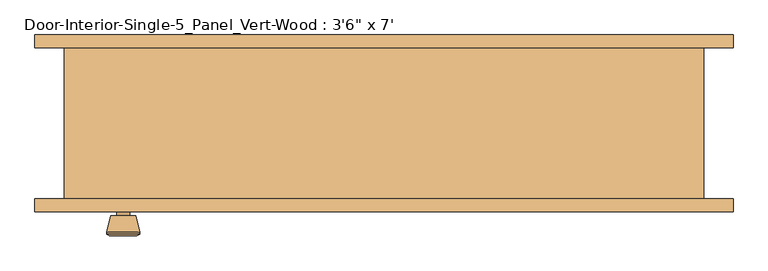
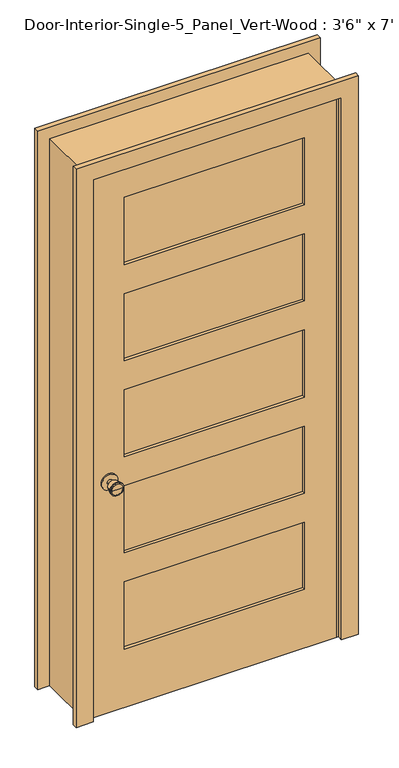
"""IFC4 building model written with IfcOpenShell, lengths in millimetres: door geometry."""

from ifc_helpers import new_model, si_unit, point, frame, frame_2d, origin, place, context, project, spatial, polyline, circle_curve, trimmed, segment, composite_curve, outline, extrude, faceted_brep, source, transform, mapped, element, save
from ifc_brep_helpers import plane_surface, cylinder_surface, revolved_surface, advanced_brep


def door_e6f20f03(model_context):
    return source(origin(), model_context, "Body", "SolidModel", [
        advanced_brep(
        [(-393.7, -70.2, 914.4), (-403.7, -70.2, 914.4), (-383.7, -70.2, 914.4), (-373.2241324, -21.2, 914.4), (-414.1758676, -21.2, 914.4), (-393.7, -21.2, 914.4), (-368.7, -23.0278681, 914.4), (-418.7, -23.0278681, 914.4), (-368.7, -26.4915463, 914.4), (-418.7, -26.4915463, 914.4), (-375.063764, -51.2, 914.4), (-412.336236, -51.2, 914.4), (-383.7, -51.2, 914.4), (-403.7, -51.2, 914.4)],
        [
            (0, 1),
            (1, 2, circle_curve(frame((-393.7, -70.2, 914.4), z_axis=(0.0, -1.0, 0.0), x_axis=(-1.0, 0.0, 0.0)), 10.0)),
            (2, 0),
            (2, 1, circle_curve(frame((-393.7, -70.2, 914.4), z_axis=(0.0, -1.0, 0.0), x_axis=(-1.0, 0.0, 0.0)), 10.0)),
            (3, 4, circle_curve(frame((-393.7, -21.2, 914.4), z_axis=(0.0, 1.0, 0.0), x_axis=(-1.0, 0.0, 0.0)), 20.4758676)),
            (4, 5),
            (5, 3),
            (4, 3, circle_curve(frame((-393.7, -21.2, 914.4), z_axis=(0.0, 1.0, 0.0), x_axis=(-1.0, 0.0, 0.0)), 20.4758676)),
            (6, 7, circle_curve(frame((-393.7, -23.0278681, 914.4), z_axis=(0.0, 1.0, 0.0), x_axis=(-1.0, 0.0, 0.0)), 25.0)),
            (7, 4),
            (3, 6),
            (7, 6, circle_curve(frame((-393.7, -23.0278681, 914.4), z_axis=(0.0, 1.0, 0.0), x_axis=(-1.0, 0.0, 0.0)), 25.0)),
            (8, 9, circle_curve(frame((-393.7, -26.4915463, 914.4), z_axis=(0.0, 1.0, 0.0), x_axis=(-1.0, 0.0, 0.0)), 25.0)),
            (9, 7),
            (6, 8),
            (9, 8, circle_curve(frame((-393.7, -26.4915463, 914.4), z_axis=(0.0, 1.0, 0.0), x_axis=(-1.0, 0.0, 0.0)), 25.0)),
            (10, 11, circle_curve(frame((-393.7, -51.2, 914.4), z_axis=(0.0, 1.0, 0.0), x_axis=(-1.0, 0.0, 0.0)), 18.636236)),
            (11, 9),
            (8, 10),
            (11, 10, circle_curve(frame((-393.7, -51.2, 914.4), z_axis=(0.0, 1.0, 0.0), x_axis=(-1.0, 0.0, 0.0)), 18.636236)),
            (12, 13, circle_curve(frame((-393.7, -51.2, 914.4), z_axis=(0.0, 1.0, 0.0), x_axis=(-1.0, 0.0, 0.0)), 10.0)),
            (13, 11),
            (10, 12),
            (13, 12, circle_curve(frame((-393.7, -51.2, 914.4), z_axis=(0.0, 1.0, 0.0), x_axis=(-1.0, 0.0, 0.0)), 10.0)),
            (1, 13),
            (12, 2),
        ],
        [
            plane_surface(frame((-393.7, -70.2, 914.4), z_axis=(0.0, -1.0, 0.0), x_axis=(-1.0, 0.0, 0.0))),
            plane_surface(frame((-393.7, -21.2, 914.4), z_axis=(0.0, 1.0, 0.0), x_axis=(-1.0, 0.0, 0.0))),
            revolved_surface(polyline([(-414.1758676, -21.2, 914.4), (-418.7, -23.0278681, 914.4)]), (-393.7, -70.2, 914.4), (0.0, -1.0, 0.0)),
            cylinder_surface(frame((-393.7, -70.2, 914.4), z_axis=(0.0, -1.0, 0.0), x_axis=(-1.0, 0.0, 0.0)), 25.0),
            revolved_surface(polyline([(-418.7, -26.4915463, 914.4), (-412.336236, -51.2, 914.4)]), (-393.7, -70.2, 914.4), (0.0, -1.0, 0.0)),
            plane_surface(frame((-393.7, -51.2, 914.4), z_axis=(0.0, -1.0, 0.0), x_axis=(-1.0, 0.0, 0.0))),
            cylinder_surface(frame((-393.7, -70.2, 914.4), z_axis=(0.0, -1.0, 0.0), x_axis=(-1.0, 0.0, 0.0)), 10.0),
        ],
        [
            (0, [[1, 2, 3]]),
            (0, [[-3, 4, -1]]),
            (1, [[5, 6, 7]]),
            (1, [[8, -7, -6]]),
            (2, [[9, 10, -5, 11]]),
            (2, [[12, -11, -8, -10]]),
            (3, [[13, 14, -9, 15]]),
            (3, [[16, -15, -12, -14]]),
            (4, [[17, 18, -13, 19]]),
            (4, [[20, -19, -16, -18]]),
            (5, [[21, 22, -17, 23]]),
            (5, [[24, -23, -20, -22]]),
            (6, [[-2, 25, -21, 26]]),
            (6, [[-4, -26, -24, -25]]),
        ],
    ),
        extrude(outline(composite_curve([segment(trimmed(circle_curve(frame_2d((914.4, -393.7)), 30.0), [point((914.4, -423.7))], [point((914.4, -363.7))], False, "CARTESIAN"), True, "CONTINUOUS"), segment(trimmed(circle_curve(frame_2d((914.4, -393.7)), 30.0), [point((914.4, -363.7))], [point((914.4, -423.7))], False, "CARTESIAN"), True, "CONTINUOUS")], self_intersect=False)), frame((0.0, -76.2, 0.0), z_axis=(0.0, 1.0, 0.0), x_axis=(0.0, 0.0, 1.0)), (0.0, 0.0, 1.0), 6.0),
        advanced_brep(
        [(-393.7, -117.125, 914.4), (-383.7, -117.125, 914.4), (-403.7, -117.125, 914.4), (-373.2241324, -166.125, 914.4), (-393.7, -166.125, 914.4), (-414.1758676, -166.125, 914.4), (-368.7, -164.2971319, 914.4), (-418.7, -164.2971319, 914.4), (-368.7, -160.8334537, 914.4), (-418.7, -160.8334537, 914.4), (-375.063764, -136.125, 914.4), (-412.336236, -136.125, 914.4), (-383.7, -136.125, 914.4), (-403.7, -136.125, 914.4)],
        [
            (0, 1),
            (1, 2, circle_curve(frame((-393.7, -117.125, 914.4), z_axis=(0.0, 1.0, 0.0), x_axis=(-1.0, 0.0, 0.0)), 10.0)),
            (2, 0),
            (2, 1, circle_curve(frame((-393.7, -117.125, 914.4), z_axis=(0.0, 1.0, 0.0), x_axis=(-1.0, 0.0, 0.0)), 10.0)),
            (3, 4),
            (4, 5),
            (5, 3, circle_curve(frame((-393.7, -166.125, 914.4), z_axis=(0.0, -1.0, 0.0), x_axis=(-1.0, 0.0, 0.0)), 20.4758676)),
            (3, 5, circle_curve(frame((-393.7, -166.125, 914.4), z_axis=(0.0, -1.0, 0.0), x_axis=(-1.0, 0.0, 0.0)), 20.4758676)),
            (6, 3),
            (5, 7),
            (7, 6, circle_curve(frame((-393.7, -164.2971319, 914.4), z_axis=(0.0, -1.0, 0.0), x_axis=(-1.0, 0.0, 0.0)), 25.0)),
            (6, 7, circle_curve(frame((-393.7, -164.2971319, 914.4), z_axis=(0.0, -1.0, 0.0), x_axis=(-1.0, 0.0, 0.0)), 25.0)),
            (8, 6),
            (7, 9),
            (9, 8, circle_curve(frame((-393.7, -160.8334537, 914.4), z_axis=(0.0, -1.0, 0.0), x_axis=(-1.0, 0.0, 0.0)), 25.0)),
            (8, 9, circle_curve(frame((-393.7, -160.8334537, 914.4), z_axis=(0.0, -1.0, 0.0), x_axis=(-1.0, 0.0, 0.0)), 25.0)),
            (10, 8),
            (9, 11),
            (11, 10, circle_curve(frame((-393.7, -136.125, 914.4), z_axis=(0.0, -1.0, 0.0), x_axis=(-1.0, 0.0, 0.0)), 18.636236)),
            (10, 11, circle_curve(frame((-393.7, -136.125, 914.4), z_axis=(0.0, -1.0, 0.0), x_axis=(-1.0, 0.0, 0.0)), 18.636236)),
            (12, 10),
            (11, 13),
            (13, 12, circle_curve(frame((-393.7, -136.125, 914.4), z_axis=(0.0, -1.0, 0.0), x_axis=(-1.0, 0.0, 0.0)), 10.0)),
            (12, 13, circle_curve(frame((-393.7, -136.125, 914.4), z_axis=(0.0, -1.0, 0.0), x_axis=(-1.0, 0.0, 0.0)), 10.0)),
            (1, 12),
            (13, 2),
        ],
        [
            plane_surface(frame((-393.7, -117.125, 914.4), z_axis=(0.0, 1.0, 0.0), x_axis=(-1.0, 0.0, 0.0))),
            plane_surface(frame((-393.7, -166.125, 914.4), z_axis=(0.0, -1.0, 0.0), x_axis=(-1.0, 0.0, 0.0))),
            revolved_surface(polyline([(-414.1758676, -166.125, 914.4), (-418.7, -164.2971319, 914.4)]), (-393.7, -117.125, 914.4), (0.0, 1.0, 0.0)),
            cylinder_surface(frame((-393.7, -117.125, 914.4), z_axis=(0.0, 1.0, 0.0), x_axis=(-1.0, 0.0, 0.0)), 25.0),
            revolved_surface(polyline([(-418.7, -160.8334537, 914.4), (-412.336236, -136.125, 914.4)]), (-393.7, -117.125, 914.4), (0.0, 1.0, 0.0)),
            plane_surface(frame((-393.7, -136.125, 914.4), z_axis=(0.0, 1.0, 0.0), x_axis=(-1.0, 0.0, 0.0))),
            cylinder_surface(frame((-393.7, -117.125, 914.4), z_axis=(0.0, 1.0, 0.0), x_axis=(-1.0, 0.0, 0.0)), 10.0),
        ],
        [
            (0, [[1, 2, 3]]),
            (0, [[-3, 4, -1]]),
            (1, [[5, 6, 7]]),
            (1, [[-6, -5, 8]]),
            (2, [[9, -7, 10, 11]]),
            (2, [[-10, -8, -9, 12]]),
            (3, [[13, -11, 14, 15]]),
            (3, [[-14, -12, -13, 16]]),
            (4, [[17, -15, 18, 19]]),
            (4, [[-18, -16, -17, 20]]),
            (5, [[21, -19, 22, 23]]),
            (5, [[-22, -20, -21, 24]]),
            (6, [[25, -23, 26, -2]]),
            (6, [[-26, -24, -25, -4]]),
        ],
    ),
        extrude(outline(composite_curve([segment(trimmed(circle_curve(frame_2d((914.4, -393.7)), 30.0), [point((914.4, -423.7))], [point((914.4, -363.7))], False, "CARTESIAN"), True, "CONTINUOUS"), segment(trimmed(circle_curve(frame_2d((914.4, -393.7)), 30.0), [point((914.4, -363.7))], [point((914.4, -423.7))], False, "CARTESIAN"), True, "CONTINUOUS")], self_intersect=False)), frame((0.0, -117.125, 0.0), z_axis=(0.0, 1.0, 0.0), x_axis=(0.0, 0.0, 1.0)), (0.0, 0.0, 1.0), 6.0),
        faceted_brep([(482.6, -111.125, 0.0), (457.2, -111.125, 0.0), (457.2, -76.2, 0.0), (444.5, -76.2, 0.0), (444.5, -41.275, 0.0), (457.2, -41.275, 0.0), (457.2, 117.475, 0.0), (482.6, 117.475, 0.0), (482.6, 117.475, 2159.0), (482.6, -111.125, 2159.0), (457.2, 117.475, 2133.6), (-457.2, 117.475, 2133.6), (-457.2, 117.475, 0.0), (-482.6, 117.475, 0.0), (-482.6, 117.475, 2159.0), (457.2, -41.275, 2133.6), (444.5, -41.275, 2120.9), (-444.5, -41.275, 2120.9), (-444.5, -41.275, 0.0), (-457.2, -41.275, 0.0), (-457.2, -41.275, 2133.6), (444.5, -76.2, 2120.9), (457.2, -76.2, 2133.6), (-457.2, -76.2, 2133.6), (-457.2, -76.2, 0.0), (-444.5, -76.2, 0.0), (-444.5, -76.2, 2120.9), (457.2, -111.125, 2133.6), (-482.6, -111.125, 2159.0), (-482.6, -111.125, 0.0), (-457.2, -111.125, 0.0), (-457.2, -111.125, 2133.6)], [[[0, 1, 2, 3, 4, 5, 6, 7]], [[7, 8, 9, 0]], [[6, 10, 11, 12, 13, 14, 8, 7]], [[5, 15, 10, 6]], [[4, 16, 17, 18, 19, 20, 15, 5]], [[3, 21, 16, 4]], [[2, 22, 23, 24, 25, 26, 21, 3]], [[1, 27, 22, 2]], [[0, 9, 28, 29, 30, 31, 27, 1]], [[8, 14, 28, 9]], [[15, 20, 11, 10]], [[21, 26, 17, 16]], [[27, 31, 23, 22]], [[29, 13, 12, 19, 18, 25, 24, 30]], [[14, 13, 29, 28]], [[20, 19, 12, 11]], [[26, 25, 18, 17]], [[31, 30, 24, 23]]]),
        extrude(outline(polyline([(2133.6, -457.2), (0.0, -457.2), (0.0, 457.2), (2133.6, 457.2), (2133.6, -457.2)]), holes=[polyline([(2014.5375, -336.55), (2014.5375, 336.55), (1749.425, 336.55), (1749.425, -336.55), (2014.5375, -336.55)]), polyline([(496.8875, -336.55), (496.8875, 336.55), (231.775, 336.55), (231.775, -336.55), (496.8875, -336.55)]), polyline([(1255.7125, -336.55), (1255.7125, 336.55), (990.6, 336.55), (990.6, -336.55), (1255.7125, -336.55)]), polyline([(1635.125, -336.55), (1635.125, 336.55), (1370.0125, 336.55), (1370.0125, -336.55), (1635.125, -336.55)]), polyline([(876.3, -336.55), (876.3, 336.55), (611.1875, 336.55), (611.1875, -336.55), (876.3, -336.55)])]), frame((0.0, -111.125, 0.0), z_axis=(0.0, 1.0, 0.0), x_axis=(0.0, 0.0, 1.0)), (0.0, 0.0, 1.0), 34.925),
        extrude(outline(polyline([(336.55, -87.8416667), (336.55, -99.4833333), (-336.55, -99.4833333), (-336.55, -87.8416667), (336.55, -87.8416667)])), frame((0.0, 0.0, 1749.425), z_axis=(0.0, 0.0, 1.0), x_axis=(1.0, 0.0, 0.0)), (0.0, 0.0, 1.0), 265.1125),
        extrude(outline(polyline([(336.55, -87.8416667), (336.55, -99.4833333), (-336.55, -99.4833333), (-336.55, -87.8416667), (336.55, -87.8416667)])), frame((0.0, 0.0, 1370.0125), z_axis=(0.0, 0.0, 1.0), x_axis=(1.0, 0.0, 0.0)), (0.0, 0.0, 1.0), 265.1125),
        extrude(outline(polyline([(336.55, -87.8416667), (336.55, -99.4833333), (-336.55, -99.4833333), (-336.55, -87.8416667), (336.55, -87.8416667)])), frame((0.0, 0.0, 611.1875), z_axis=(0.0, 0.0, 1.0), x_axis=(1.0, 0.0, 0.0)), (0.0, 0.0, 1.0), 265.1125),
        extrude(outline(polyline([(336.55, -87.8416667), (336.55, -99.4833333), (-336.55, -99.4833333), (-336.55, -87.8416667), (336.55, -87.8416667)])), frame((0.0, 0.0, 231.775), z_axis=(0.0, 0.0, 1.0), x_axis=(1.0, 0.0, 0.0)), (0.0, 0.0, 1.0), 265.1125),
        extrude(outline(polyline([(336.55, -87.8416667), (336.55, -99.4833333), (-336.55, -99.4833333), (-336.55, -87.8416667), (336.55, -87.8416667)])), frame((0.0, 0.0, 990.6), z_axis=(0.0, 0.0, 1.0), x_axis=(1.0, 0.0, 0.0)), (0.0, 0.0, 1.0), 265.1125),
        extrude(outline(polyline([(0.0, 527.05), (2203.45, 527.05), (2203.45, -527.05), (0.0, -527.05), (0.0, -463.55), (2139.95, -463.55), (2139.95, 463.55), (0.0, 463.55), (0.0, 527.05)])), frame((0.0, -130.175, 0.0), z_axis=(0.0, 1.0, 0.0), x_axis=(0.0, 0.0, 1.0)), (0.0, 0.0, 1.0), 19.05),
        extrude(outline(polyline([(0.0, 527.05), (2203.45, 527.05), (2203.45, -527.05), (0.0, -527.05), (0.0, -463.55), (2139.95, -463.55), (2139.95, 463.55), (0.0, 463.55), (0.0, 527.05)])), frame((0.0, 117.475, 0.0), z_axis=(0.0, 1.0, 0.0), x_axis=(0.0, 0.0, 1.0)), (0.0, 0.0, 1.0), 19.05),
    ])


if __name__ == "__main__":
    model = new_model("IFC4")
    model_context = context("Model", 3, world=origin())
    ifc_project = project(units=[si_unit("LENGTHUNIT", "METRE", prefix="MILLI")], contexts=[model_context])
    site = spatial("IfcSite", under=ifc_project)
    building = spatial("IfcBuilding", under=site)
    placement = place(None, origin())
    door_shape = door_e6f20f03(model_context)
    element("IfcDoor", 1, ObjectType="Door-Interior-Single-5_Panel_Vert-Wood : 3'6\" x 7'", at=placement, inside=building, context=model_context, shape_type="MappedRepresentation", body=[
        mapped(door_shape, transform((0.0, 0.0, 0.0), x_axis=(1.0, 0.0, 0.0), y_axis=(0.0, 1.0, 0.0), z_axis=(0.0, 0.0, 1.0))),
    ])
    save(model, "model.ifc")

# Revit data of these elements
# Type "Door-Interior-Single-5_Panel_Vert-Wood : 3'6\" x 7'"
#   Type Mark = "9"
#   Assembly Code = "C1020300"
#   Analytic Construction = "Wooden"
#   Top Rail = 0' - 4 11/16"
#   Thickness = 0' - 1 3/8"
#   Thermal Resistance (R) = 2.5876 (h·ft²·°F)/BTU
#   Swing Angle [instance default] = 90.00°
#   Stiles = 0' - 4 3/4"
#   Rough Width = 3' - 2"
#   Rough Height = 7' - 1"
#   Intermediate Rail = 0' - 4 1/2"
#   Height = 7' - 0"
#   Width = 3' - 0"
#   Heat Transfer Coefficient (U) = 0.3865 BTU/(h·ft²·°F)
#   Bottom Rail = 0' - 9 1/8"
#   Trim Material = DOOR 1
#   Panel Material = DOOR 1
#   Frame Material = DOOR 1
#   Door Handle Material = Aluminum
#   Visual Light Transmittance = 0
#   Solar Heat Gain Coefficient = 0
#   Wall Closure = (empty or 0)
#   Function = (empty or 0)
# Element 1 (IfcDoor, "Door-Interior-Single-5_Panel_Vert-Wood : 3'6\" x 7'")
#   Materials on its faces: "DOOR 1", "Aluminum"
# Materials
#   "DOOR 1": class "Generic", colour RGB 120 120 120, transparency 0, Cost = 0
#   "Aluminum": class "Metal", colour RGB 247 247 247, transparency 0, Description = "Aluminum 6061", Cost = 0
